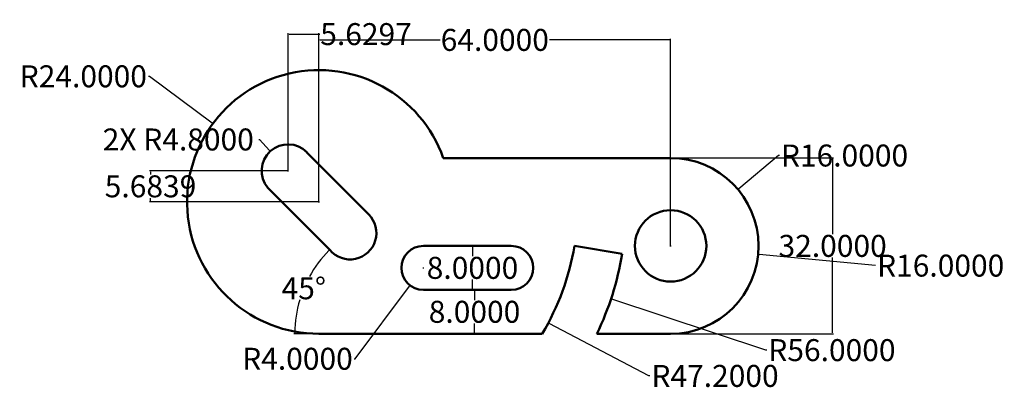
# Model space of a CAD drawing. Units: inches. Extents: x 248 to 427, y 128 to 195.
import ezdxf

# ---------------------------------------------------------------- set-up
doc = ezdxf.new("R2010")
doc.units = ezdxf.units.IN
doc.header["$MEASUREMENT"] = 0
doc.layers.add('M-DIMS', color=2, linetype='Continuous', lineweight=25)
doc.layers.add('M-OUTL', color=7, linetype='Continuous', lineweight=50)
doc.styles.get("Standard").update_dxf_attribs({"font": 'arial.ttf'})
doc.dimstyles.get("Standard").update_dxf_attribs({"dimtxt": 4, "dimasz": 0.18, "dimexe": 0.18, "dimexo": 0.0625, "dimgap": 0.09, "dimtad": 0, "dimtih": 1, "dimtoh": 1, "dimdec": 4, "dimzin": 0, "dimdsep": 46, "dimtxsty": 'Standard', "dimcen": 0.09, "dimadec": 0, "dimazin": 0, "dimtfac": 1, "dimtdec": 4, "dimtofl": 0, "dimtmove": 0, "dimatfit": 3, "dimfxl": 1, "dimtolj": 1, "dimtzin": 0, "dimarcsym": 0})

# ---------------------------------------------------------------- blocks, each defined once
blk = doc.blocks.new('*D1')
at = {"layer": 'Defpoints', "color": 0, "transparency": 16777216}
for p in [(302.41, 191.79), (302.41, 162.29), (366.41, 154.29)]:
    blk.add_point(p, dxfattribs=at)
at = {"layer": 'M-DIMS', "color": 0, "lineweight": -2, "transparency": 16777216}
for p, q in [((302.41, 162.35), (302.41, 191.97)), ((302.59, 191.79), (324.46, 191.79)), ((366.23, 191.79), (344.36, 191.79)), ((366.41, 154.35), (366.41, 191.97))]:
    blk.add_line(p, q, dxfattribs=at)
at = {"layer": 'M-DIMS', "color": 0, "transparency": 16777216}
for points in [[(302.59, 191.82), (302.59, 191.76), (302.41, 191.79)], [(366.23, 191.82), (366.23, 191.76), (366.41, 191.79)]]:
    blk.add_solid(points, dxfattribs=at)
at = {"layer": 'M-DIMS', "color": 0, "transparency": 16777216, "insert": (334.41, 191.79), "char_height": 4, "attachment_point": 5}
blk.add_mtext('\\A1;64.0000', dxfattribs=at)
blk = doc.blocks.new('*D2')
at = {"layer": 'Defpoints', "color": 0, "transparency": 16777216}
for p in [(321.41, 150.29), (319.01, 147.09)]:
    blk.add_point(p, dxfattribs=at)
at = {"layer": 'M-DIMS', "color": 0, "lineweight": -2, "transparency": 16777216}
for p, q in [((321.32, 150.29), (321.5, 150.29)), ((321.41, 150.2), (321.41, 150.38)), ((308.98, 133.74), (318.9, 146.95)), ((308.8, 133.74), (308.98, 133.74))]:
    blk.add_line(p, q, dxfattribs=at)
at = {"layer": 'M-DIMS', "color": 0, "transparency": 16777216}
blk.add_solid([(318.87, 146.96), (318.92, 146.93), (319.01, 147.09)], dxfattribs=at)
at = {"layer": 'M-DIMS', "color": 0, "transparency": 16777216, "insert": (298.5, 133.74), "char_height": 4, "attachment_point": 5}
blk.add_mtext('\\A1;R4.0000', dxfattribs=at)
blk = doc.blocks.new('*D3')
at = {"layer": 'Defpoints', "color": 0, "transparency": 16777216}
for p in [(302.41, 162.29), (355.56, 144.65)]:
    blk.add_point(p, dxfattribs=at)
at = {"layer": 'M-DIMS', "color": 0, "lineweight": -2, "transparency": 16777216}
for p, q in [((302.32, 162.29), (302.5, 162.29)), ((302.41, 162.2), (302.41, 162.38)), ((383.72, 135.31), (355.73, 144.59)), ((383.9, 135.31), (383.72, 135.31))]:
    blk.add_line(p, q, dxfattribs=at)
at = {"layer": 'M-DIMS', "color": 0, "transparency": 16777216}
blk.add_solid([(355.74, 144.62), (355.72, 144.57), (355.56, 144.65)], dxfattribs=at)
at = {"layer": 'M-DIMS', "color": 0, "transparency": 16777216, "insert": (395.76, 135.31), "char_height": 4, "attachment_point": 5}
blk.add_mtext('\\A1;R56.0000', dxfattribs=at)
blk = doc.blocks.new('*D4')
at = {"layer": 'Defpoints', "color": 0, "transparency": 16777216}
for p in [(366.41, 154.29), (382.34, 152.76)]:
    blk.add_point(p, dxfattribs=at)
at = {"layer": 'M-DIMS', "color": 0, "lineweight": -2, "transparency": 16777216}
for p, q in [((366.32, 154.29), (366.5, 154.29)), ((366.41, 154.2), (366.41, 154.38)), ((403.7, 150.7), (382.51, 152.74))]:
    blk.add_line(p, q, dxfattribs=at)
at = {"layer": 'M-DIMS', "color": 0, "transparency": 16777216}
blk.add_solid([(382.52, 152.77), (382.51, 152.71), (382.34, 152.76)], dxfattribs=at)
at = {"layer": 'M-DIMS', "color": 0, "transparency": 16777216, "insert": (415.55, 150.7), "char_height": 4, "attachment_point": 5}
blk.add_mtext('\\A1;R16.0000', dxfattribs=at)
blk = doc.blocks.new('*D5')
at = {"layer": 'Defpoints', "color": 0, "transparency": 16777216}
for p in [(302.41, 162.29), (344.16, 140.27)]:
    blk.add_point(p, dxfattribs=at)
at = {"layer": 'M-DIMS', "color": 0, "lineweight": -2, "transparency": 16777216}
for p, q in [((302.32, 162.29), (302.5, 162.29)), ((302.41, 162.2), (302.41, 162.38)), ((362.45, 130.62), (344.32, 140.19)), ((362.63, 130.62), (362.45, 130.62))]:
    blk.add_line(p, q, dxfattribs=at)
at = {"layer": 'M-DIMS', "color": 0, "transparency": 16777216}
blk.add_solid([(344.33, 140.21), (344.3, 140.16), (344.16, 140.27)], dxfattribs=at)
at = {"layer": 'M-DIMS', "color": 0, "transparency": 16777216, "insert": (374.49, 130.62), "char_height": 4, "attachment_point": 5}
blk.add_mtext('\\A1;R47.2000', dxfattribs=at)
blk = doc.blocks.new('*D6')
at = {"layer": 'Defpoints', "color": 0, "transparency": 16777216}
for p in [(329.41, 154.29), (329.41, 146.29), (330.35, 146.29)]:
    blk.add_point(p, dxfattribs=at)
at = {"layer": 'M-DIMS', "color": 0, "lineweight": -2, "transparency": 16777216}
for p, q in [((329.47, 154.29), (330.53, 154.29)), ((330.35, 154.11), (330.35, 152.42)), ((330.35, 146.47), (330.35, 148.15)), ((329.47, 146.29), (330.53, 146.29))]:
    blk.add_line(p, q, dxfattribs=at)
at = {"layer": 'M-DIMS', "color": 0, "transparency": 16777216}
for points in [[(330.32, 154.11), (330.38, 154.11), (330.35, 154.29)], [(330.32, 146.47), (330.38, 146.47), (330.35, 146.29)]]:
    blk.add_solid(points, dxfattribs=at)
at = {"layer": 'M-DIMS', "color": 0, "transparency": 16777216, "insert": (330.35, 150.29), "char_height": 4, "attachment_point": 5}
blk.add_mtext('\\A1;8.0000', dxfattribs=at)
blk = doc.blocks.new('*D7')
at = {"layer": 'Defpoints', "color": 0, "transparency": 16777216}
for p in [(330.35, 146.29), (330.35, 138.29), (330.72, 138.29)]:
    blk.add_point(p, dxfattribs=at)
at = {"layer": 'M-DIMS', "color": 0, "lineweight": -2, "transparency": 16777216}
for p, q in [((330.41, 146.29), (330.9, 146.29)), ((330.72, 146.11), (330.72, 144.42)), ((330.72, 138.47), (330.72, 140.15)), ((330.41, 138.29), (330.9, 138.29))]:
    blk.add_line(p, q, dxfattribs=at)
at = {"layer": 'M-DIMS', "color": 0, "transparency": 16777216}
for points in [[(330.69, 146.11), (330.75, 146.11), (330.72, 146.29)], [(330.69, 138.47), (330.75, 138.47), (330.72, 138.29)]]:
    blk.add_solid(points, dxfattribs=at)
at = {"layer": 'M-DIMS', "color": 0, "transparency": 16777216, "insert": (330.72, 142.29), "char_height": 4, "attachment_point": 5}
blk.add_mtext('\\A1;8.0000', dxfattribs=at)
blk = doc.blocks.new('*D8')
at = {"layer": 'Defpoints', "color": 0, "transparency": 16777216}
for p in [(298.73, 159.2), (304.39, 153.54), (300.9, 149.11), (302.41, 138.29), (321.41, 138.29)]:
    blk.add_point(p, dxfattribs=at)
at = {"layer": 'M-DIMS', "color": 0, "lineweight": -2, "transparency": 16777216}
blk.add_line((302.35, 138.29), (297.82, 138.29), dxfattribs=at)
for start, end in [(135.4765, 151.2603), (163.4689, 179.5235)]:
    blk.add_arc((319.65, 138.29), 21.64, start, end, dxfattribs=at)
at = {"layer": 'M-DIMS', "color": 0, "transparency": 16777216}
for points in [[(304.19, 153.48), (304.24, 153.44), (304.34, 153.59)], [(298.03, 138.47), (297.97, 138.47), (298, 138.29)]]:
    blk.add_solid(points, dxfattribs=at)
at = {"layer": 'M-DIMS', "color": 0, "transparency": 16777216, "insert": (299.65, 146.57), "char_height": 4, "attachment_point": 5}
blk.add_mtext('\\A1;45°', dxfattribs=at)
blk = doc.blocks.new('*D9')
at = {"layer": 'Defpoints', "color": 0, "transparency": 16777216}
for p in [(366.41, 170.29), (366.41, 138.29), (395.89, 138.29)]:
    blk.add_point(p, dxfattribs=at)
at = {"layer": 'M-DIMS', "color": 0, "lineweight": -2, "transparency": 16777216}
for p, q in [((366.47, 170.29), (396.07, 170.29)), ((395.89, 170.11), (395.89, 156.42)), ((395.89, 138.47), (395.89, 152.15)), ((366.47, 138.29), (396.07, 138.29))]:
    blk.add_line(p, q, dxfattribs=at)
at = {"layer": 'M-DIMS', "color": 0, "transparency": 16777216}
for points in [[(395.86, 170.11), (395.92, 170.11), (395.89, 170.29)], [(395.86, 138.47), (395.92, 138.47), (395.89, 138.29)]]:
    blk.add_solid(points, dxfattribs=at)
at = {"layer": 'M-DIMS', "color": 0, "transparency": 16777216, "insert": (395.89, 154.29), "char_height": 4, "attachment_point": 5}
blk.add_mtext('\\A1;32.0000', dxfattribs=at)
blk = doc.blocks.new('*D10')
at = {"layer": 'Defpoints', "color": 0, "transparency": 16777216}
for p in [(302.41, 192.84), (296.78, 167.97), (302.41, 162.29)]:
    blk.add_point(p, dxfattribs=at)
at = {"layer": 'M-DIMS', "color": 0, "lineweight": -2, "transparency": 16777216}
for p, q in [((296.78, 168.03), (296.78, 193.02)), ((296.96, 192.84), (302.23, 192.84)), ((302.41, 162.35), (302.41, 193.02)), ((302.41, 192.84), (302.59, 192.84))]:
    blk.add_line(p, q, dxfattribs=at)
at = {"layer": 'M-DIMS', "color": 0, "transparency": 16777216}
for points in [[(296.96, 192.87), (296.96, 192.81), (296.78, 192.84)], [(302.23, 192.87), (302.23, 192.81), (302.41, 192.84)]]:
    blk.add_solid(points, dxfattribs=at)
at = {"layer": 'M-DIMS', "color": 0, "transparency": 16777216, "insert": (310.98, 192.84), "char_height": 4, "attachment_point": 5}
blk.add_mtext('\\A1;5.6297', dxfattribs=at)
blk = doc.blocks.new('*D11')
at = {"layer": 'Defpoints', "color": 0, "transparency": 16777216}
for p in [(296.78, 167.97), (271.76, 162.29), (302.41, 162.29)]:
    blk.add_point(p, dxfattribs=at)
at = {"layer": 'M-DIMS', "color": 0, "lineweight": -2, "transparency": 16777216}
for p, q in [((296.72, 167.97), (271.58, 167.97)), ((271.76, 167.79), (271.76, 167.26)), ((302.35, 162.29), (271.58, 162.29)), ((271.76, 162.47), (271.76, 163))]:
    blk.add_line(p, q, dxfattribs=at)
at = {"layer": 'M-DIMS', "color": 0, "transparency": 16777216}
for points in [[(271.73, 167.79), (271.79, 167.79), (271.76, 167.97)], [(271.73, 162.47), (271.79, 162.47), (271.76, 162.29)]]:
    blk.add_solid(points, dxfattribs=at)
at = {"layer": 'M-DIMS', "color": 0, "transparency": 16777216, "insert": (271.76, 165.13), "char_height": 4, "attachment_point": 5}
blk.add_mtext('\\A1;5.6839', dxfattribs=at)
blk = doc.blocks.new('*D12')
at = {"layer": 'Defpoints', "color": 0, "transparency": 16777216}
for p in [(283.13, 176.58), (302.41, 162.29)]:
    blk.add_point(p, dxfattribs=at)
at = {"layer": 'M-DIMS', "color": 0, "lineweight": -2, "transparency": 16777216}
for p, q in [((271.38, 185.16), (271.56, 185.16)), ((271.56, 185.16), (282.98, 176.69)), ((302.32, 162.29), (302.5, 162.29)), ((302.41, 162.2), (302.41, 162.38))]:
    blk.add_line(p, q, dxfattribs=at)
at = {"layer": 'M-DIMS', "color": 0, "transparency": 16777216}
blk.add_solid([(283, 176.71), (282.97, 176.66), (283.13, 176.58)], dxfattribs=at)
at = {"layer": 'M-DIMS', "color": 0, "transparency": 16777216, "insert": (259.53, 185.16), "char_height": 4, "attachment_point": 5}
blk.add_mtext('\\A1;R24.0000', dxfattribs=at)
blk = doc.blocks.new('*D13')
at = {"layer": 'Defpoints', "color": 0, "transparency": 16777216}
for p in [(378.67, 164.57), (366.41, 154.29)]:
    blk.add_point(p, dxfattribs=at)
at = {"layer": 'M-DIMS', "color": 0, "lineweight": -2, "transparency": 16777216}
for p, q in [((386.02, 170.74), (378.8, 164.69)), ((386.2, 170.74), (386.02, 170.74)), ((366.32, 154.29), (366.5, 154.29)), ((366.41, 154.2), (366.41, 154.38))]:
    blk.add_line(p, q, dxfattribs=at)
at = {"layer": 'M-DIMS', "color": 0, "transparency": 16777216}
blk.add_solid([(378.78, 164.71), (378.82, 164.66), (378.67, 164.57)], dxfattribs=at)
at = {"layer": 'M-DIMS', "color": 0, "transparency": 16777216, "insert": (398.05, 170.74), "char_height": 4, "attachment_point": 5}
blk.add_mtext('\\A1;R16.0000', dxfattribs=at)
blk = doc.blocks.new('*D14')
at = {"layer": 'Defpoints', "color": 0, "transparency": 16777216}
for p in [(293.55, 171.53), (296.78, 167.97)]:
    blk.add_point(p, dxfattribs=at)
at = {"layer": 'M-DIMS', "color": 0, "lineweight": -2, "transparency": 16777216}
for p, q in [((291.44, 173.66), (291.62, 173.66)), ((291.62, 173.66), (293.43, 171.66)), ((296.69, 167.97), (296.87, 167.97)), ((296.78, 167.88), (296.78, 168.06))]:
    blk.add_line(p, q, dxfattribs=at)
at = {"layer": 'M-DIMS', "color": 0, "transparency": 16777216}
blk.add_solid([(293.45, 171.68), (293.41, 171.64), (293.55, 171.53)], dxfattribs=at)
at = {"layer": 'M-DIMS', "color": 0, "transparency": 16777216, "insert": (276.81, 173.66), "char_height": 4, "attachment_point": 5}
blk.add_mtext('\\A1;2X R4.8000', dxfattribs=at)

msp = doc.modelspace()

# ---------------------------------------------------------------- linework, layer by layer
at = {"layer": 'M-OUTL'}
for p, q in [((305.80264, 165.68126), (300.17296, 171.36517)), ((325.03594, 170.28715), (366.40852, 170.28715)), ((298.73151, 159.20177), (293.10184, 164.88567)), ((305.80264, 165.68126), (311.45949, 160.02441)), ((298.73151, 159.20177), (304.38836, 153.54491)), ((321.40852, 154.28715), (337.40852, 154.28715)), ((348.92562, 154.28715), (357.60365, 152.82681)), ((321.40852, 146.28715), (337.40852, 146.28715)), ((302.40852, 138.28715), (321.40852, 138.28715)), ((321.40852, 138.28715), (343.05136, 138.28715)), ((353.00497, 138.28715), (366.40852, 138.28715))]:
    msp.add_line(p, q, dxfattribs=at)
msp.add_circle((366.40852, 154.28715), 6.5, dxfattribs=at)
for centre, radius, start, end in [((302.40852, 162.28715), 24, 19.4712206, 270), ((296.77885, 167.97105), 4.8, 44.4506559, 220), ((366.40852, 154.28715), 16, 270, 90), ((308.06538, 156.63029), 4.8, 220, 45), ((321.40852, 150.28715), 4, 90, 270), ((337.40852, 150.28715), 4, 270, 90), ((302.40852, 162.28715), 47.2, 329.4377246, 350.2417434), ((302.40852, 162.28715), 56, 334.6230665, 350.2741189)]:
    msp.add_arc(centre, radius, start, end, dxfattribs=at)

# ---------------------------------------------------------------- dimensions: what is measured, and where the dimension line sits
at = {"layer": 'M-DIMS'}
for base, p1, override, picture, middle in [((302.40852, 192.84446), (296.77885, 167.97106), {"dimdec": 4, "dimlfac": 1, "dimrnd": 0, "dimzin": 0, "dimdsep": 46, "dimlunit": 2}, '*D10', (310.98139, 192.84446)), ((302.40852, 191.79053), (366.40852, 154.28715), {"dimclrd": 0, "dimclre": 0, "dimclrt": 0}, '*D1', (334.40852, 191.79053))]:
    dim = msp.add_linear_dim(base=base, p1=p1, p2=(302.40852, 162.28715), dimstyle='Standard', override=override, dxfattribs=at)
    dim.commit()
    dim.dimension.update_dxf_attribs({"geometry": picture, "text_midpoint": middle})
for center, mpoint, override, picture, middle in [((302.40852, 162.28715), (283.12911, 176.58066), {"dimdec": 4, "dimlfac": 1, "dimrnd": 0, "dimzin": 0, "dimdsep": 46, "dimlunit": 2}, '*D12', (259.52749, 185.15676)), ((366.40852, 154.28715), (378.66501, 164.57201), {"dimdec": 4, "dimlfac": 1, "dimrnd": 0, "dimzin": 0, "dimdsep": 46, "dimlunit": 2}, '*D13', (398.05289, 170.74293)), ((302.40852, 162.28715), (355.55909, 144.65147), {"dimclrd": 0, "dimclre": 0, "dimclrt": 0}, '*D3', (395.7566, 135.30664)), ((302.40852, 162.28715), (344.1584, 140.26925), {"dimclrd": 0, "dimclre": 0, "dimclrt": 0}, '*D5', (374.4854, 130.62195)), ((366.40852, 154.28715), (382.335, 152.75505), {"dimclrd": 0, "dimclre": 0, "dimclrt": 0}, '*D4', (403.70025, 150.69976)), ((321.40852, 150.28715), (319.00583, 147.08917), {"dimclrd": 0, "dimclre": 0, "dimclrt": 0}, '*D2', (298.49519, 133.73858))]:
    dim = msp.add_radius_dim(center=center, mpoint=mpoint, dimstyle='Standard', override=override, dxfattribs=at)
    dim.commit()
    dim.dimension.update_dxf_attribs({"geometry": picture, "text_midpoint": middle, "dimtype": 164})
dim = msp.add_radius_dim(center=(296.77885, 167.97106), mpoint=(293.55277, 171.52526), text='2X <>', dimstyle='Standard', override={"dimdec": 4, "dimlfac": 1, "dimrnd": 0, "dimzin": 0, "dimdsep": 46, "dimlunit": 2}, dxfattribs=at)
dim.commit()
dim.dimension.update_dxf_attribs({"geometry": '*D14', "text_midpoint": (276.8055, 173.65778), "dimtype": 164})
for base, p1, p2, override, picture, middle in [((395.88979, 138.28715), (366.40852, 170.28715), (366.40852, 138.28715), {"dimclrd": 0, "dimclre": 0, "dimclrt": 0}, '*D9', (395.88979, 154.28715)), ((271.76234, 162.28715), (296.77885, 167.97106), (302.40852, 162.28715), {"dimdec": 4, "dimlfac": 1, "dimrnd": 0, "dimzin": 0, "dimdsep": 46, "dimlunit": 2}, '*D11', (271.76234, 165.1291)), ((330.34993, 146.28715), (329.40852, 154.28715), (329.40852, 146.28715), {"dimclrd": 0, "dimclre": 0, "dimclrt": 0}, '*D6', (330.34993, 150.28715)), ((330.71581, 138.28715), (330.34993, 146.28715), (330.34993, 138.28715), {"dimclrd": 0, "dimclre": 0, "dimclrt": 0}, '*D7', (330.71581, 142.28715))]:
    dim = msp.add_linear_dim(base=base, p1=p1, p2=p2, angle=90, dimstyle='Standard', override=override, dxfattribs=at)
    dim.commit()
    dim.dimension.update_dxf_attribs({"geometry": picture, "text_midpoint": middle})
dim = msp.add_angular_dim_2l(base=(300.90368, 149.1081), line1=((302.40852, 138.28715), (321.40852, 138.28715)), line2=((298.73151, 159.20177), (304.38836, 153.54491)), dimstyle='Standard', override={"dimclrd": 0, "dimclre": 0, "dimclrt": 0}, dxfattribs=at)
dim.commit()
dim.dimension.update_dxf_attribs({"geometry": '*D8', "text_midpoint": (299.65161, 146.56915)})

doc.saveas('drawing.dxf')
